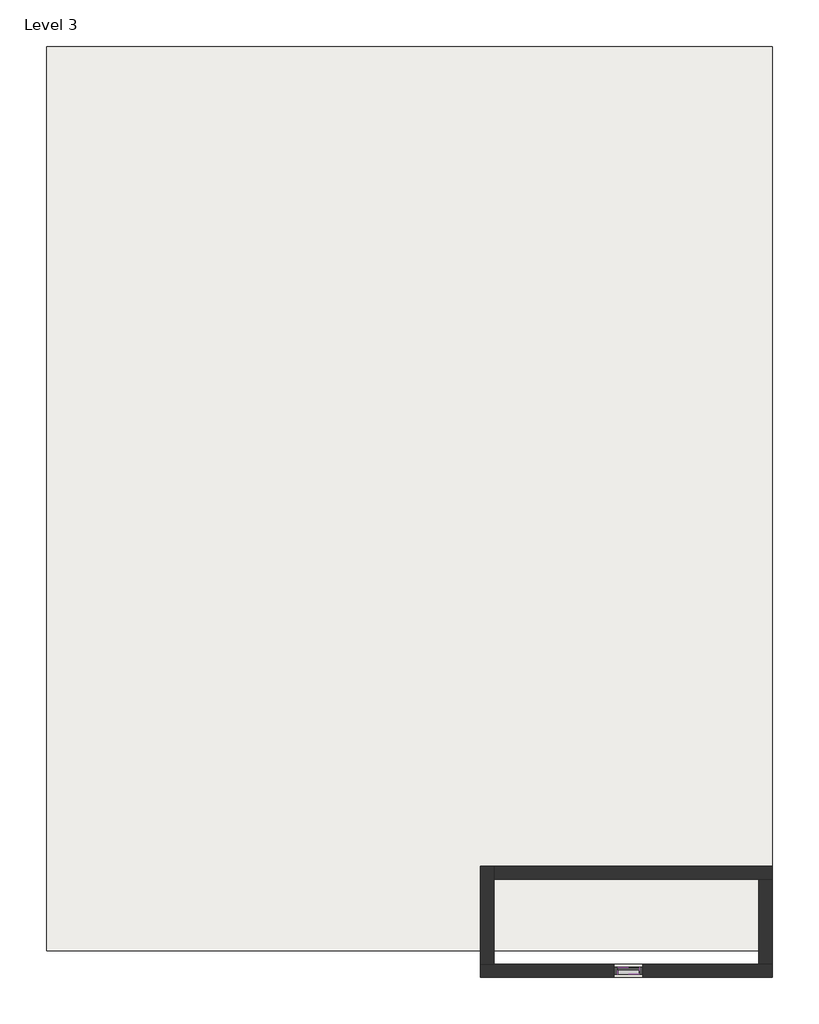
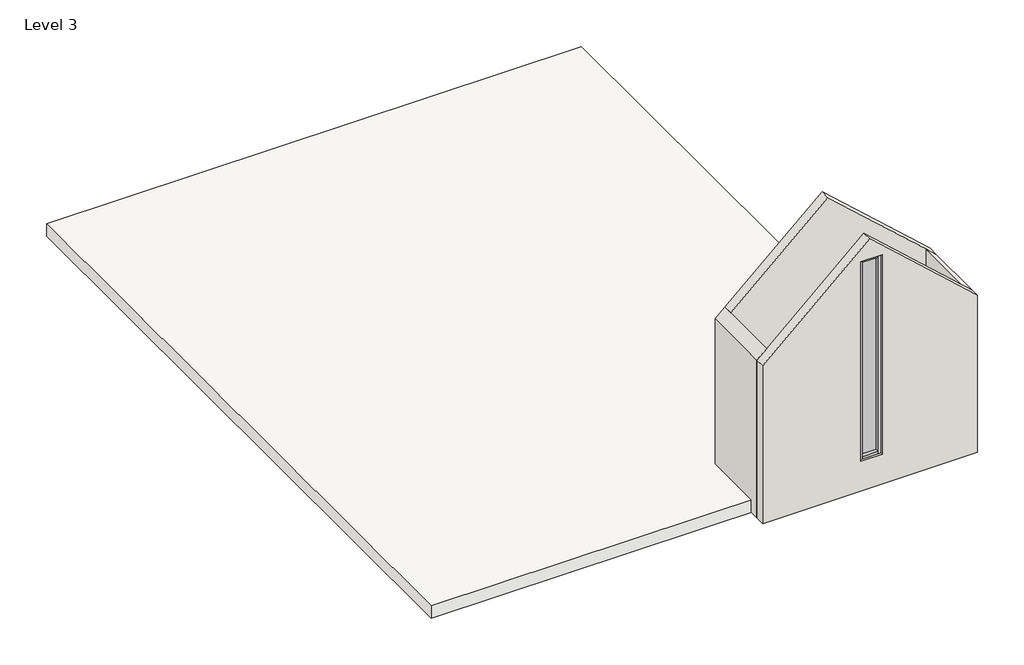
# One storey: 4 members, 4 walls, 1 plate, 1 roof.
"""IFC4 building model written with IfcOpenShell, lengths in millimetres."""

from ifc_helpers import new_model, si_unit, frame, origin, place, context, project, spatial, polyline, outline, extrude, faceted_brep, transform, mapped, element, save
from components import member_83c59054, member_8d537d56, system_panel_glazed_557308a9

model = new_model("IFC4")

# Units and contexts
model_context = context("Model", 3, world=origin())
ifc_project = project(units=[si_unit("LENGTHUNIT", "METRE", prefix="MILLI")], contexts=[model_context])

# Site, building, storey
site = spatial("IfcSite", under=ifc_project)
building = spatial("IfcBuilding", under=site)
storey = spatial("IfcBuildingStorey", under=building, Name="Level 3", Elevation=6096.0)

# Members
placement = place(None, origin())
member_shape = member_83c59054(model_context)
element("IfcMember", 1, ObjectType="Rectangular Mullion : 2.5\" x 5\" rectangular", at=placement, inside=storey, context=model_context, shape_type="MappedRepresentation", body=[
    mapped(member_shape, transform((-6075.7859258, -12143.9777232, 11719.6239199), x_axis=(0.0, 0.0, 1.0), y_axis=(0.0, -1.0, 0.0), z_axis=(1.0, 0.0, 0.0))),
])
element("IfcMember", 2, ObjectType="Rectangular Mullion : 2.5\" x 5\" rectangular", at=placement, inside=storey, context=model_context, shape_type="MappedRepresentation", body=[
    mapped(member_shape, transform((-6444.0859258, -12143.9777232, 6824.3067345), x_axis=(0.0, 0.0, -1.0), y_axis=(0.0, -1.0, 0.0), z_axis=(-1.0, 0.0, 0.0))),
])
member_2_shape = member_8d537d56(model_context)
element("IfcMember", 3, ObjectType="Rectangular Mullion : 2.5\" x 5\" rectangular", at=placement, inside=storey, context=model_context, shape_type="MappedRepresentation", body=[
    mapped(member_2_shape, transform((-6012.2859258, -12143.9777232, 6824.3067345), x_axis=(1.0, 0.0, 0.0), y_axis=(0.0, -1.0, 0.0), z_axis=(0.0, 0.0, -1.0))),
])
element("IfcMember", 4, ObjectType="Rectangular Mullion : 2.5\" x 5\" rectangular", at=placement, inside=storey, context=model_context, shape_type="MappedRepresentation", body=[
    mapped(member_2_shape, transform((-6507.5859258, -12143.9777232, 11719.6239199), x_axis=(-1.0, 0.0, 0.0), y_axis=(0.0, -1.0, 0.0), z_axis=(0.0, 0.0, 1.0))),
])

# Plate
system_panel_glazed_shape = system_panel_glazed_557308a9(model_context)
element("IfcPlate", 5, ObjectType="System Panel : Glazed", at=placement, inside=storey, context=model_context, shape_type="MappedRepresentation", body=[
    mapped(system_panel_glazed_shape, transform((-6259.9359258, -12143.9777232, 6887.8067345), x_axis=(1.0, 0.0, 0.0), y_axis=(0.0, 1.0, 0.0), z_axis=(0.0, 0.0, 1.0))),
])

# Roof
element("IfcRoof", 6, ObjectType="Generic - 12\"", at=placement, inside=storey, context=model_context, shape_type="SweptSolid", body=[
    extrude(outline(polyline([(-16223.0859258, 3667.5222768), (-3802.4859258, 3667.5222768), (-3802.4859258, -11801.0777232), (-16223.0859258, -11801.0777232), (-16223.0859258, 3667.5222768)])), frame((0.0, 0.0, 6096.0), z_axis=(0.0, 0.0, 1.0), x_axis=(1.0, 0.0, 0.0)), (0.0, 0.0, 1.0), 304.8),
])

# Walls
element("IfcWall", 7, ObjectType="9\"", at=placement, inside=storey, context=model_context, shape_type="Brep", body=[
    faceted_brep([(-3802.4859258, -12029.6777232, 6096.0), (-4031.0859258, -12029.6777232, 6096.0), (-8564.9859258, -12029.6777232, 6096.0), (-8793.5859258, -12029.6777232, 6096.0), (-8793.5859258, -12029.6777232, 9965.817204), (-8564.9859258, -12029.6777232, 10172.4964728), (-6308.1216094, -12029.6777232, 12212.9473328), (-4031.0859258, -12029.6777232, 10154.2593625), (-3802.4859258, -12029.6777232, 9947.5800938), (-6507.5859258, -12029.6777232, 11719.6239199), (-6507.5859258, -12029.6777232, 6824.3067345), (-6012.2859258, -12029.6777232, 6824.3067345), (-6012.2859258, -12029.6777232, 11719.6239199), (-8793.5859258, -12258.2777232, 6096.0), (-3802.4859258, -12258.2777232, 6096.0), (-3802.4859258, -12258.2777232, 9947.5800938), (-6308.1216094, -12258.2777232, 12212.9473328), (-8793.5859258, -12258.2777232, 9965.817204), (-6507.5859258, -12258.2777232, 6824.3067345), (-6507.5859258, -12258.2777232, 11719.6239199), (-6012.2859258, -12258.2777232, 11719.6239199), (-6012.2859258, -12258.2777232, 6824.3067345)], [[[0, 1, 2, 3, 4, 5, 6, 7, 8], [9, 10, 11, 12]], [[13, 14, 15, 16, 17], [18, 19, 20, 21]], [[3, 2, 1, 0, 14, 13]], [[4, 3, 13, 17]], [[0, 8, 15, 14]], [[15, 8, 7, 6, 16]], [[4, 17, 16, 6, 5]], [[18, 10, 9, 19]], [[19, 9, 12, 20]], [[20, 12, 11, 21]], [[10, 18, 21, 11]]]),
])
element("IfcWall", 8, ObjectType="9\"", at=placement, inside=storey, context=model_context, shape_type="Brep", body=[
    faceted_brep([(-8564.9859258, -12029.6777232, 6096.0), (-8564.9859258, -10581.8777232, 6096.0), (-8564.9859258, -10353.2777232, 6096.0), (-8564.9859258, -10353.2777232, 10172.4964728), (-8564.9859258, -10581.8777232, 10172.4964728), (-8564.9859258, -12029.6777232, 10172.4964728), (-8793.5859258, -12029.6777232, 6096.0), (-8793.5859258, -12029.6777232, 9965.817204), (-8793.5859258, -10353.2777232, 9965.817204), (-8793.5859258, -10353.2777232, 6096.0)], [[[0, 1, 2, 3, 4, 5]], [[6, 7, 8, 9]], [[2, 1, 0, 6, 9]], [[0, 5, 7, 6]], [[3, 2, 9, 8]], [[5, 4, 3, 8, 7]]]),
])
element("IfcWall", 9, ObjectType="9\"", at=placement, inside=storey, context=model_context, shape_type="Brep", body=[
    faceted_brep([(-8564.9859258, -10581.8777232, 6096.0), (-4031.0859258, -10581.8777232, 6096.0), (-3802.4859258, -10581.8777232, 6096.0), (-3802.4859258, -10581.8777232, 9947.5800938), (-4031.0859258, -10581.8777232, 10154.2593625), (-6308.1216094, -10581.8777232, 12212.9473328), (-8564.9859258, -10581.8777232, 10172.4964728), (-8564.9859258, -10353.2777232, 6096.0), (-8564.9859258, -10353.2777232, 10172.4964728), (-6308.1216094, -10353.2777232, 12212.9473328), (-3802.4859258, -10353.2777232, 9947.5800938), (-3802.4859258, -10353.2777232, 6096.0)], [[[0, 1, 2, 3, 4, 5, 6]], [[7, 8, 9, 10, 11]], [[2, 1, 0, 7, 11]], [[0, 6, 8, 7]], [[3, 2, 11, 10]], [[6, 5, 9, 8]], [[5, 4, 3, 10, 9]]]),
])
element("IfcWall", 10, ObjectType="9\"", at=placement, inside=storey, context=model_context, shape_type="SweptSolid", body=[
    extrude(outline(polyline([(10154.2593625, -4031.0859258), (6096.0, -4031.0859258), (6096.0, -3802.4859258), (9947.5800938, -3802.4859258), (10154.2593625, -4031.0859258)])), frame((0.0, -12029.6777232, 0.0), z_axis=(0.0, 1.0, 0.0), x_axis=(0.0, 0.0, 1.0)), (0.0, 0.0, 1.0), 1447.8),
])

save(model, "model.ifc")

# Revit data of these elements
# Type "Rectangular Mullion : 2.5\" x 5\" rectangular"
#   built-in parameter 1007304 = 0.416667 (stored number, unit not read)
#   built-in parameter 1007301 = 0.104167 (stored number, unit not read)
#   built-in parameter 1007300 = 0.104167 (stored number, unit not read)
# Type "System Panel : Glazed"
#   Construction Type Id = "GSP4R"
#   Analytic Construction = "1/8 in Pilkington single glazing"
#   Visual Light Transmittance = 0.9
#   Solar Heat Gain Coefficient = 0.86
#   Heat Transfer Coefficient (U) = 1.18115 BTU/(h·ft²·°F)
#   Define Thermal Properties by = 1
# Type "Generic - 12\""
#   Assembly Code = "B1020"
#   Layers, outside or top first: 1' - 0" no material (function 1)
# Type "9\""
#   Assembly Code = "B2010"
#   Layers, outside or top first: 0' - 9" no material (function 1)
# Elements 1, 2, 3, 4 (IfcMember, "Rectangular Mullion : 2.5\" x 5\" rectangular")
#   Phase Created = New Construction
#   Materials on its faces: "Aluminum"
# Element 5 (IfcPlate, "System Panel : Glazed")
#   Phase Created = New Construction
#   Materials on its faces: "Glass"
# Element 6 (IfcRoof, "Generic - 12\"")
#   built-in parameter 1001705 = 21 (stored number, unit not read)
#   built-in parameter 1001710 = 33615
#   Phase Created = New Construction
#   Materials on its faces: "Default Roof"
# Elements 7, 8, 9, 10 (IfcWall, "9\"")
#   Top Offset = 0' - 0"
#   Base Offset = 0' - 0"
#   Unconnected Height = 10' - 0"
#   wall height = 10' - 0"
#   Phase Created = New Construction
#   Base Constraint = Level 3
#   Materials on its faces: "Default Wall"
# Materials
#   "Aluminum": class "Metal", colour RGB 247 247 247, transparency 0, Description = "Aluminum 6061", Cost = 0
#   "Glass": class "Glass", colour RGB 0 128 192, transparency 0.75, Description = "Soda Lime Glass", Cost = 0
#   "Default Roof": colour RGB 88 101 114, transparency 0, Cost = 0
#   "Default Wall": colour RGB 128 128 128, transparency 0, Cost = 0
